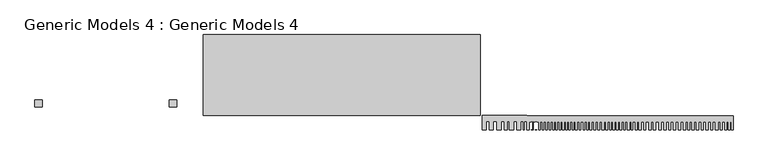
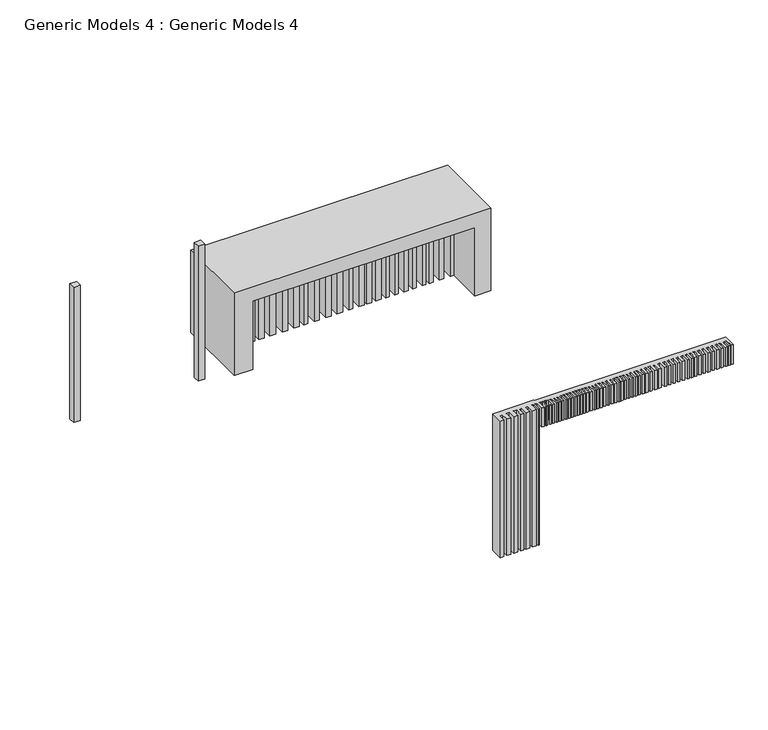
"""IFC4 building model written with IfcOpenShell, lengths in millimetres: proxy geometry, Generic Models 4 : Generic Models 4."""

from ifc_helpers import new_model, si_unit, frame, origin, place, context, project, spatial, polyline, outline, extrude, faceted_brep, source, transform, mapped, element, save


def generic_models_4_generic_models_4_29f9d9a5(model_context):
    return source(origin(), model_context, "Body", "SolidModel", [
        faceted_brep([(-8072.8951638, -14169.1466243, 3352.8), (-8072.8951638, -14169.1466243, 2880.6848502), (-8019.8245913, -14169.1466243, 2880.6848502), (-8019.8245913, -14169.1466243, 3352.8), (-3625.114323, -14169.1466243, 2880.6848502), (-3625.114323, -14169.1466243, 3352.8), (-3665.2507979, -14169.1466243, 3352.8), (-3665.2507979, -14169.1466243, 2880.6848502), (-7933.2939962, -14169.1466243, 3352.8), (-7974.3314326, -14169.1466243, 3352.8), (-7974.3314326, -14169.1466243, 2880.6848502), (-7933.2939962, -14169.1466243, 2880.6848502), (-7780.27289, -14169.1466243, 3352.8), (-7815.2998882, -14169.1466243, 3352.8), (-7815.2998882, -14169.1466243, 2880.6848502), (-7780.27289, -14169.1466243, 2880.6848502), (-7702.1357404, -14169.1466243, 3352.8), (-7737.1627385, -14169.1466243, 3352.8), (-7737.1627385, -14169.1466243, 2880.6848502), (-7702.1357404, -14169.1466243, 2880.6848502), (-7629.3873597, -14169.1466243, 3352.8), (-7664.4143578, -14169.1466243, 3352.8), (-7664.4143578, -14169.1466243, 2880.6848502), (-7629.3873597, -14169.1466243, 2880.6848502), (-7559.3333635, -14169.1466243, 3352.8), (-7591.6659771, -14169.1466243, 3352.8), (-7591.6659771, -14169.1466243, 2880.6848502), (-7559.3333635, -14169.1466243, 2880.6848502), (-7478.5018294, -14169.1466243, 3352.8), (-7516.223212, -14169.1466243, 3352.8), (-7516.223212, -14169.1466243, 2880.6848502), (-7478.5018294, -14169.1466243, 2880.6848502), (-7411.1422177, -14169.1466243, 3352.8), (-7443.4748313, -14169.1466243, 3352.8), (-7443.4748313, -14169.1466243, 2880.6848502), (-7411.1422177, -14169.1466243, 2880.6848502), (-7343.7826059, -14169.1466243, 3352.8), (-7376.1152195, -14169.1466243, 3352.8), (-7376.1152195, -14169.1466243, 2880.6848502), (-7343.7826059, -14169.1466243, 2880.6848502), (-7265.6454563, -14169.1466243, 3352.8), (-7308.7556078, -14169.1466243, 3352.8), (-7308.7556078, -14169.1466243, 2880.6848502), (-7265.6454563, -14169.1466243, 2880.6848502), (-7203.6746135, -14169.1466243, 3352.8), (-7236.0072271, -14169.1466243, 3352.8), (-7236.0072271, -14169.1466243, 2880.6848502), (-7203.6746135, -14169.1466243, 2880.6848502), (-7133.6206172, -14169.1466243, 3352.8), (-7165.9532309, -14169.1466243, 3352.8), (-7165.9532309, -14169.1466243, 2880.6848502), (-7133.6206172, -14169.1466243, 2880.6848502), (-7058.1778521, -14169.1466243, 3352.8), (-7093.2048502, -14169.1466243, 3352.8), (-7093.2048502, -14169.1466243, 2880.6848502), (-7058.1778521, -14169.1466243, 2880.6848502), (-6980.0407025, -14169.1466243, 3352.8), (-7023.150854, -14169.1466243, 3352.8), (-7023.150854, -14169.1466243, 2880.6848502), (-6980.0407025, -14169.1466243, 2880.6848502), (-6904.5979373, -14169.1466243, 3352.8), (-6942.3193199, -14169.1466243, 3352.8), (-6942.3193199, -14169.1466243, 2880.6848502), (-6904.5979373, -14169.1466243, 2880.6848502), (-6823.7664032, -14169.1466243, 3352.8), (-6858.7934013, -14169.1466243, 3352.8), (-6858.7934013, -14169.1466243, 2880.6848502), (-6823.7664032, -14169.1466243, 2880.6848502), (-6748.323638, -14169.1466243, 3352.8), (-6783.3506361, -14169.1466243, 3352.8), (-6783.3506361, -14169.1466243, 2880.6848502), (-6748.323638, -14169.1466243, 2880.6848502), (-6672.8808729, -14169.1466243, 3352.8), (-6710.6022555, -14169.1466243, 3352.8), (-6710.6022555, -14169.1466243, 2880.6848502), (-6672.8808729, -14169.1466243, 2880.6848502), (-6589.3549543, -14169.1466243, 3352.8), (-6627.0763369, -14169.1466243, 3352.8), (-6627.0763369, -14169.1466243, 2880.6848502), (-6589.3549543, -14169.1466243, 2880.6848502), (-6503.1346513, -14169.1466243, 3352.8), (-6543.5504183, -14169.1466243, 3352.8), (-6543.5504183, -14169.1466243, 2880.6848502), (-6503.1346513, -14169.1466243, 2880.6848502), (-6406.1368103, -14169.1466243, 3352.8), (-6454.6357308, -14169.1466243, 3352.8), (-6454.6357308, -14169.1466243, 2880.6848502), (-6406.1368103, -14169.1466243, 2880.6848502), (-6328.4825754, -14169.1466243, 3352.8), (-6371.1098122, -14169.1466243, 3352.8), (-6371.1098122, -14169.1466243, 2880.6848502), (-6328.4825754, -14169.1466243, 2880.6848502), (-6249.8625111, -14169.1466243, 3352.8), (-6284.8895092, -14169.1466243, 3352.8), (-6284.8895092, -14169.1466243, 2880.6848502), (-6249.8625111, -14169.1466243, 2880.6848502), (-6174.4197459, -14169.1466243, 3352.8), (-6220.2242819, -14169.1466243, 3352.8), (-6220.2242819, -14169.1466243, 2880.6848502), (-6174.4197459, -14169.1466243, 2880.6848502), (-6104.3657497, -14169.1466243, 3352.8), (-6139.3927478, -14169.1466243, 3352.8), (-6139.3927478, -14169.1466243, 2880.6848502), (-6104.3657497, -14169.1466243, 2880.6848502), (-6023.5342156, -14169.1466243, 3352.8), (-6066.6443671, -14169.1466243, 3352.8), (-6066.6443671, -14169.1466243, 2880.6848502), (-6023.5342156, -14169.1466243, 2880.6848502), (-5948.0914504, -14169.1466243, 3352.8), (-5983.1184486, -14169.1466243, 3352.8), (-5983.1184486, -14169.1466243, 2880.6848502), (-5948.0914504, -14169.1466243, 2880.6848502), (-5849.0047434, -14169.1466243, 3352.8), (-5904.9812989, -14169.1466243, 3352.8), (-5904.9812989, -14169.1466243, 2880.6848502), (-5849.0047434, -14169.1466243, 2880.6848502), (-5783.7339978, -14169.1466243, 3352.8), (-5818.7609959, -14169.1466243, 3352.8), (-5818.7609959, -14169.1466243, 2880.6848502), (-5783.7339978, -14169.1466243, 2880.6848502), (-5694.8193103, -14169.1466243, 3352.8), (-5735.2350773, -14169.1466243, 3352.8), (-5735.2350773, -14169.1466243, 2880.6848502), (-5694.8193103, -14169.1466243, 2880.6848502), (-5600.5748667, -14169.1466243, 3352.8), (-5654.4035432, -14169.1466243, 3352.8), (-5654.4035432, -14169.1466243, 2880.6848502), (-5600.5748667, -14169.1466243, 2880.6848502), (-5508.6233048, -14169.1466243, 3352.8), (-5551.3831863, -14169.1466243, 3352.8), (-5551.3831863, -14169.1466243, 2880.6848502), (-5508.6233048, -14169.1466243, 2880.6848502), (-5391.0336306, -14169.1466243, 3352.8), (-5444.4834825, -14169.1466243, 3352.8), (-5444.4834825, -14169.1466243, 2880.6848502), (-5391.0336306, -14169.1466243, 2880.6848502), (-5291.2605737, -14169.1466243, 3352.8), (-5348.273749, -14169.1466243, 3352.8), (-5348.273749, -14169.1466243, 2880.6848502), (-5291.2605737, -14169.1466243, 2880.6848502), (-5170.107576, -14169.1466243, 3352.8), (-5230.6840748, -14169.1466243, 3352.8), (-5230.6840748, -14169.1466243, 2880.6848502), (-5170.107576, -14169.1466243, 2880.6848502), (-5070.334519, -14169.1466243, 3352.8), (-5116.657724, -14169.1466243, 3352.8), (-5116.657724, -14169.1466243, 2880.6848502), (-5070.334519, -14169.1466243, 2880.6848502), (-4966.9981386, -14169.1466243, 3352.8), (-5013.3213436, -14169.1466243, 3352.8), (-5013.3213436, -14169.1466243, 2880.6848502), (-4966.9981386, -14169.1466243, 2880.6848502), (-4860.0984348, -14169.1466243, 3352.8), (-4909.9849633, -14169.1466243, 3352.8), (-4909.9849633, -14169.1466243, 2880.6848502), (-4860.0984348, -14169.1466243, 2880.6848502), (-4753.198731, -14169.1466243, 3352.8), (-4806.6485829, -14169.1466243, 3352.8), (-4806.6485829, -14169.1466243, 2880.6848502), (-4753.198731, -14169.1466243, 2880.6848502), (-4649.8623506, -14169.1466243, 3352.8), (-4696.1855556, -14169.1466243, 3352.8), (-4696.1855556, -14169.1466243, 2880.6848502), (-4649.8623506, -14169.1466243, 2880.6848502), (-4553.6526171, -14169.1466243, 3352.8), (-4603.5391456, -14169.1466243, 3352.8), (-4603.5391456, -14169.1466243, 2880.6848502), (-4553.6526171, -14169.1466243, 2880.6848502), (-4464.5695306, -14169.1466243, 3352.8), (-4510.8927356, -14169.1466243, 3352.8), (-4510.8927356, -14169.1466243, 2880.6848502), (-4464.5695306, -14169.1466243, 2880.6848502), (-4364.7964736, -14169.1466243, 3352.8), (-4418.2463256, -14169.1466243, 3352.8), (-4418.2463256, -14169.1466243, 2880.6848502), (-4364.7964736, -14169.1466243, 2880.6848502), (-4268.5867402, -14169.1466243, 3352.8), (-4314.9099452, -14169.1466243, 3352.8), (-4314.9099452, -14169.1466243, 2880.6848502), (-4268.5867402, -14169.1466243, 2880.6848502), (-4158.1237129, -14169.1466243, 3352.8), (-4218.7002117, -14169.1466243, 3352.8), (-4218.7002117, -14169.1466243, 2880.6848502), (-4158.1237129, -14169.1466243, 2880.6848502), (-4058.350656, -14169.1466243, 3352.8), (-4104.673861, -14169.1466243, 3352.8), (-4104.673861, -14169.1466243, 2880.6848502), (-4058.350656, -14169.1466243, 2880.6848502), (-3947.8876286, -14169.1466243, 3352.8), (-4004.900804, -14169.1466243, 3352.8), (-4004.900804, -14169.1466243, 2880.6848502), (-3947.8876286, -14169.1466243, 2880.6848502), (-3853.714323, -14169.1466243, 3352.8), (-3899.240517, -14169.1466243, 3352.8), (-3899.240517, -14169.1466243, 2880.6848502), (-3853.714323, -14169.1466243, 2880.6848502), (-3766.003205, -14169.1466243, 3352.8), (-3809.382795, -14169.1466243, 3352.8), (-3809.382795, -14169.1466243, 2880.6848502), (-3766.003205, -14169.1466243, 2880.6848502), (-3688.6802281, -14169.1466243, 3352.8), (-3725.7221572, -14169.1466243, 3352.8), (-3725.7221572, -14169.1466243, 2880.6848502), (-3688.6802281, -14169.1466243, 2880.6848502), (-3625.114323, -13864.3466243, 3352.8), (-3625.114323, -13864.3466243, 2880.6848502), (-8072.8951638, -13864.3466243, 2880.6848502), (-8072.8951638, -13864.3466243, 3352.8), (-8072.8951638, -13854.1538163, 3352.8), (-9031.8508279, -13854.1538163, 3352.8), (-9031.8508279, -14158.9538163, 3352.8), (-8947.3984101, -14158.9538163, 3352.8), (-8947.3984101, -13981.1538163, 3352.8), (-8878.843385, -13981.1538163, 3352.8), (-8878.843385, -14158.9538163, 3352.8), (-8791.591535, -14158.9538163, 3352.8), (-8791.591535, -13981.1538163, 3352.8), (-8723.0365099, -13981.1538163, 3352.8), (-8723.0365099, -14158.9538163, 3352.8), (-8623.3201098, -14158.9538163, 3352.8), (-8623.3201098, -13981.1538163, 3352.8), (-8552.3729958, -13981.1538163, 3352.8), (-8552.3729958, -14158.9538163, 3352.8), (-8491.4762732, -14158.9538163, 3352.8), (-8491.4762732, -13981.1538163, 3352.8), (-8443.291009, -13981.1538163, 3352.8), (-8443.291009, -14158.9538163, 3352.8), (-8349.8068839, -14158.9538163, 3352.8), (-8349.8068839, -13981.1538163, 3352.8), (-8287.4841338, -13981.1538163, 3352.8), (-8287.4841338, -14158.9538163, 3352.8), (-8200.8633881, -14158.9538163, 3352.8), (-8200.8633881, -13981.1538163, 3352.8), (-8151.7037606, -13981.1538163, 3352.8), (-8151.7037606, -14158.9538163, 3352.8), (-8123.0396657, -14158.9538163, 3352.8), (-8123.0396657, -13981.1538163, 3352.8), (-8072.8951638, -13981.1538163, 3352.8), (-8019.8245913, -13981.1538163, 3352.8), (-8009.5759038, -13981.1538163, 3352.8), (-8009.5759038, -13991.3466243, 3352.8), (-8001.1139413, -13991.3466243, 3352.8), (-8001.1139413, -13981.1538163, 3352.8), (-7990.6394273, -13981.1538163, 3352.8), (-7990.6394273, -13991.3466243, 3352.8), (-7974.3314326, -13991.3466243, 3352.8), (-7974.3314326, -13981.1538163, 3352.8), (-7946.1776726, -13981.1538163, 3352.8), (-7946.1776726, -14158.9538163, 3352.8), (-7974.3314326, -14158.9538163, 3352.8), (-7933.2939962, -13981.1538163, 3352.8), (-7908.7622496, -13981.1538163, 3352.8), (-7908.7622496, -13991.3466243, 3352.8), (-7885.3328194, -13991.3466243, 3352.8), (-7885.3328194, -13981.1538163, 3352.8), (-7854.214323, -13981.1538163, 3352.8), (-7854.214323, -13991.3466243, 3352.8), (-7815.2998882, -13991.3466243, 3352.8), (-7780.27289, -13991.3466243, 3352.8), (-7737.1627385, -13991.3466243, 3352.8), (-7702.1357404, -13991.3466243, 3352.8), (-7664.4143578, -13991.3466243, 3352.8), (-7629.3873597, -13991.3466243, 3352.8), (-7591.6659771, -13991.3466243, 3352.8), (-7559.3333635, -13991.3466243, 3352.8), (-7516.223212, -13991.3466243, 3352.8), (-7478.5018294, -13991.3466243, 3352.8), (-7443.4748313, -13991.3466243, 3352.8), (-7411.1422177, -13991.3466243, 3352.8), (-7376.1152195, -13991.3466243, 3352.8), (-7343.7826059, -13991.3466243, 3352.8), (-7308.7556078, -13991.3466243, 3352.8), (-7265.6454563, -13991.3466243, 3352.8), (-7236.0072271, -13991.3466243, 3352.8), (-7203.6746135, -13991.3466243, 3352.8), (-7165.9532309, -13991.3466243, 3352.8), (-7133.6206172, -13991.3466243, 3352.8), (-7093.2048502, -13991.3466243, 3352.8), (-7058.1778521, -13991.3466243, 3352.8), (-7023.150854, -13991.3466243, 3352.8), (-6980.0407025, -13991.3466243, 3352.8), (-6942.3193199, -13991.3466243, 3352.8), (-6904.5979373, -13991.3466243, 3352.8), (-6858.7934013, -13991.3466243, 3352.8), (-6823.7664032, -13991.3466243, 3352.8), (-6783.3506361, -13991.3466243, 3352.8), (-6748.323638, -13991.3466243, 3352.8), (-6710.6022555, -13991.3466243, 3352.8), (-6672.8808729, -13991.3466243, 3352.8), (-6627.0763369, -13991.3466243, 3352.8), (-6589.3549543, -13991.3466243, 3352.8), (-6543.5504183, -13991.3466243, 3352.8), (-6503.1346513, -13991.3466243, 3352.8), (-6454.6357308, -13991.3466243, 3352.8), (-6406.1368103, -13991.3466243, 3352.8), (-6371.1098122, -13991.3466243, 3352.8), (-6328.4825754, -13991.3466243, 3352.8), (-6284.8895092, -13991.3466243, 3352.8), (-6249.8625111, -13991.3466243, 3352.8), (-6220.2242819, -13991.3466243, 3352.8), (-6174.4197459, -13991.3466243, 3352.8), (-6139.3927478, -13991.3466243, 3352.8), (-6104.3657497, -13991.3466243, 3352.8), (-6066.6443671, -13991.3466243, 3352.8), (-6023.5342156, -13991.3466243, 3352.8), (-5983.1184486, -13991.3466243, 3352.8), (-5948.0914504, -13991.3466243, 3352.8), (-5904.9812989, -13991.3466243, 3352.8), (-5849.0047434, -13991.3466243, 3352.8), (-5818.7609959, -13991.3466243, 3352.8), (-5783.7339978, -13991.3466243, 3352.8), (-5735.2350773, -13991.3466243, 3352.8), (-5694.8193103, -13991.3466243, 3352.8), (-5654.4035432, -13991.3466243, 3352.8), (-5600.5748667, -13991.3466243, 3352.8), (-5551.3831863, -13991.3466243, 3352.8), (-5508.6233048, -13991.3466243, 3352.8), (-5444.4834825, -13991.3466243, 3352.8), (-5391.0336306, -13991.3466243, 3352.8), (-5348.273749, -13991.3466243, 3352.8), (-5291.2605737, -13991.3466243, 3352.8), (-5230.6840748, -13991.3466243, 3352.8), (-5170.107576, -13991.3466243, 3352.8), (-5116.657724, -13991.3466243, 3352.8), (-5070.334519, -13991.3466243, 3352.8), (-5013.3213436, -13991.3466243, 3352.8), (-4966.9981386, -13991.3466243, 3352.8), (-4909.9849633, -13991.3466243, 3352.8), (-4860.0984348, -13991.3466243, 3352.8), (-4806.6485829, -13991.3466243, 3352.8), (-4753.198731, -13991.3466243, 3352.8), (-4696.1855556, -13991.3466243, 3352.8), (-4649.8623506, -13991.3466243, 3352.8), (-4603.5391456, -13991.3466243, 3352.8), (-4553.6526171, -13991.3466243, 3352.8), (-4510.8927356, -13991.3466243, 3352.8), (-4464.5695306, -13991.3466243, 3352.8), (-4418.2463256, -13991.3466243, 3352.8), (-4364.7964736, -13991.3466243, 3352.8), (-4314.9099452, -13991.3466243, 3352.8), (-4268.5867402, -13991.3466243, 3352.8), (-4218.7002117, -13991.3466243, 3352.8), (-4158.1237129, -13991.3466243, 3352.8), (-4104.673861, -13991.3466243, 3352.8), (-4058.350656, -13991.3466243, 3352.8), (-4004.900804, -13991.3466243, 3352.8), (-3947.8876286, -13991.3466243, 3352.8), (-3899.240517, -13991.3466243, 3352.8), (-3853.714323, -13991.3466243, 3352.8), (-3809.382795, -13991.3466243, 3352.8), (-3766.003205, -13991.3466243, 3352.8), (-3725.7221572, -13991.3466243, 3352.8), (-3688.6802281, -13991.3466243, 3352.8), (-3665.2507979, -13991.3466243, 3352.8), (-8072.8951638, -13981.1538163, 2880.6848502), (-3665.2507979, -13991.3466243, 2880.6848502), (-3688.6802281, -13991.3466243, 2880.6848502), (-3725.7221572, -13991.3466243, 2880.6848502), (-3766.003205, -13991.3466243, 2880.6848502), (-3809.382795, -13991.3466243, 2880.6848502), (-3853.714323, -13991.3466243, 2880.6848502), (-3899.240517, -13991.3466243, 2880.6848502), (-3947.8876286, -13991.3466243, 2880.6848502), (-4004.900804, -13991.3466243, 2880.6848502), (-4058.350656, -13991.3466243, 2880.6848502), (-4104.673861, -13991.3466243, 2880.6848502), (-4158.1237129, -13991.3466243, 2880.6848502), (-4218.7002117, -13991.3466243, 2880.6848502), (-4268.5867402, -13991.3466243, 2880.6848502), (-4314.9099452, -13991.3466243, 2880.6848502), (-4364.7964736, -13991.3466243, 2880.6848502), (-4418.2463256, -13991.3466243, 2880.6848502), (-4464.5695306, -13991.3466243, 2880.6848502), (-4510.8927356, -13991.3466243, 2880.6848502), (-4553.6526171, -13991.3466243, 2880.6848502), (-4603.5391456, -13991.3466243, 2880.6848502), (-4649.8623506, -13991.3466243, 2880.6848502), (-4696.1855556, -13991.3466243, 2880.6848502), (-4753.198731, -13991.3466243, 2880.6848502), (-4806.6485829, -13991.3466243, 2880.6848502), (-4860.0984348, -13991.3466243, 2880.6848502), (-4909.9849633, -13991.3466243, 2880.6848502), (-4966.9981386, -13991.3466243, 2880.6848502), (-5013.3213436, -13991.3466243, 2880.6848502), (-5070.334519, -13991.3466243, 2880.6848502), (-5116.657724, -13991.3466243, 2880.6848502), (-5170.107576, -13991.3466243, 2880.6848502), (-5230.6840748, -13991.3466243, 2880.6848502), (-5291.2605737, -13991.3466243, 2880.6848502), (-5348.273749, -13991.3466243, 2880.6848502), (-5391.0336306, -13991.3466243, 2880.6848502), (-5444.4834825, -13991.3466243, 2880.6848502), (-5508.6233048, -13991.3466243, 2880.6848502), (-5551.3831863, -13991.3466243, 2880.6848502), (-5600.5748667, -13991.3466243, 2880.6848502), (-5654.4035432, -13991.3466243, 2880.6848502), (-5694.8193103, -13991.3466243, 2880.6848502), (-5735.2350773, -13991.3466243, 2880.6848502), (-5783.7339978, -13991.3466243, 2880.6848502), (-5818.7609959, -13991.3466243, 2880.6848502), (-5849.0047434, -13991.3466243, 2880.6848502), (-5904.9812989, -13991.3466243, 2880.6848502), (-5948.0914504, -13991.3466243, 2880.6848502), (-5983.1184486, -13991.3466243, 2880.6848502), (-6023.5342156, -13991.3466243, 2880.6848502), (-6066.6443671, -13991.3466243, 2880.6848502), (-6104.3657497, -13991.3466243, 2880.6848502), (-6139.3927478, -13991.3466243, 2880.6848502), (-6174.4197459, -13991.3466243, 2880.6848502), (-6220.2242819, -13991.3466243, 2880.6848502), (-6249.8625111, -13991.3466243, 2880.6848502), (-6284.8895092, -13991.3466243, 2880.6848502), (-6328.4825754, -13991.3466243, 2880.6848502), (-6371.1098122, -13991.3466243, 2880.6848502), (-6406.1368103, -13991.3466243, 2880.6848502), (-6454.6357308, -13991.3466243, 2880.6848502), (-6503.1346513, -13991.3466243, 2880.6848502), (-6543.5504183, -13991.3466243, 2880.6848502), (-6589.3549543, -13991.3466243, 2880.6848502), (-6627.0763369, -13991.3466243, 2880.6848502), (-6672.8808729, -13991.3466243, 2880.6848502), (-6710.6022555, -13991.3466243, 2880.6848502), (-6748.323638, -13991.3466243, 2880.6848502), (-6783.3506361, -13991.3466243, 2880.6848502), (-6823.7664032, -13991.3466243, 2880.6848502), (-6858.7934013, -13991.3466243, 2880.6848502), (-6904.5979373, -13991.3466243, 2880.6848502), (-6942.3193199, -13991.3466243, 2880.6848502), (-6980.0407025, -13991.3466243, 2880.6848502), (-7023.150854, -13991.3466243, 2880.6848502), (-7058.1778521, -13991.3466243, 2880.6848502), (-7093.2048502, -13991.3466243, 2880.6848502), (-7133.6206172, -13991.3466243, 2880.6848502), (-7165.9532309, -13991.3466243, 2880.6848502), (-7203.6746135, -13991.3466243, 2880.6848502), (-7236.0072271, -13991.3466243, 2880.6848502), (-7265.6454563, -13991.3466243, 2880.6848502), (-7308.7556078, -13991.3466243, 2880.6848502), (-7343.7826059, -13991.3466243, 2880.6848502), (-7376.1152195, -13991.3466243, 2880.6848502), (-7411.1422177, -13991.3466243, 2880.6848502), (-7443.4748313, -13991.3466243, 2880.6848502), (-7478.5018294, -13991.3466243, 2880.6848502), (-7516.223212, -13991.3466243, 2880.6848502), (-7559.3333635, -13991.3466243, 2880.6848502), (-7591.6659771, -13991.3466243, 2880.6848502), (-7629.3873597, -13991.3466243, 2880.6848502), (-7664.4143578, -13991.3466243, 2880.6848502), (-7702.1357404, -13991.3466243, 2880.6848502), (-7737.1627385, -13991.3466243, 2880.6848502), (-7780.27289, -13991.3466243, 2880.6848502), (-7815.2998882, -13991.3466243, 2880.6848502), (-7854.214323, -13991.3466243, 2880.6848502), (-7854.214323, -13981.1538163, 2880.6848502), (-7885.3328194, -13981.1538163, 2880.6848502), (-7885.3328194, -13991.3466243, 2880.6848502), (-7908.7622496, -13991.3466243, 2880.6848502), (-7908.7622496, -13981.1538163, 2880.6848502), (-7933.2939962, -13981.1538163, 2880.6848502), (-7974.3314326, -14158.9538163, 2880.6848502), (-7946.1776726, -14158.9538163, 2880.6848502), (-7946.1776726, -13981.1538163, 2880.6848502), (-7974.3314326, -13981.1538163, 2880.6848502), (-7974.3314326, -13991.3466243, 2880.6848502), (-7990.6394273, -13991.3466243, 2880.6848502), (-7990.6394273, -13981.1538163, 2880.6848502), (-8001.1139413, -13981.1538163, 2880.6848502), (-8001.1139413, -13991.3466243, 2880.6848502), (-8009.5759038, -13991.3466243, 2880.6848502), (-8009.5759038, -13981.1538163, 2880.6848502), (-8019.8245913, -13981.1538163, 2880.6848502), (-9031.8508279, -14158.9538163, 0.0), (-8947.3984101, -14158.9538163, 0.0), (-8151.7037606, -14158.9538163, 0.0), (-8123.0396657, -14158.9538163, 0.0), (-8287.4841338, -14158.9538163, 0.0), (-8200.8633881, -14158.9538163, 0.0), (-8443.291009, -14158.9538163, 0.0), (-8349.8068839, -14158.9538163, 0.0), (-8552.3729958, -14158.9538163, 0.0), (-8491.4762732, -14158.9538163, 0.0), (-8723.0365099, -14158.9538163, 0.0), (-8623.3201098, -14158.9538163, 0.0), (-8878.843385, -14158.9538163, 0.0), (-8791.591535, -14158.9538163, 0.0), (-9031.8508279, -13854.1538163, 0.0), (-8072.8951638, -13854.1538163, 0.0), (-8072.8951638, -13981.1538163, 0.0), (-8123.0396657, -13981.1538163, 0.0), (-8151.7037606, -13981.1538163, 0.0), (-8200.8633881, -13981.1538163, 0.0), (-8287.4841338, -13981.1538163, 0.0), (-8349.8068839, -13981.1538163, 0.0), (-8443.291009, -13981.1538163, 0.0), (-8491.4762732, -13981.1538163, 0.0), (-8552.3729958, -13981.1538163, 0.0), (-8623.3201098, -13981.1538163, 0.0), (-8723.0365099, -13981.1538163, 0.0), (-8791.591535, -13981.1538163, 0.0), (-8878.843385, -13981.1538163, 0.0), (-8947.3984101, -13981.1538163, 0.0)], [[[0, 1, 2, 3]], [[4, 5, 6, 7]], [[8, 9, 10, 11]], [[12, 13, 14, 15]], [[16, 17, 18, 19]], [[20, 21, 22, 23]], [[24, 25, 26, 27]], [[28, 29, 30, 31]], [[32, 33, 34, 35]], [[36, 37, 38, 39]], [[40, 41, 42, 43]], [[44, 45, 46, 47]], [[48, 49, 50, 51]], [[52, 53, 54, 55]], [[56, 57, 58, 59]], [[60, 61, 62, 63]], [[64, 65, 66, 67]], [[68, 69, 70, 71]], [[72, 73, 74, 75]], [[76, 77, 78, 79]], [[80, 81, 82, 83]], [[84, 85, 86, 87]], [[88, 89, 90, 91]], [[92, 93, 94, 95]], [[96, 97, 98, 99]], [[100, 101, 102, 103]], [[104, 105, 106, 107]], [[108, 109, 110, 111]], [[112, 113, 114, 115]], [[116, 117, 118, 119]], [[120, 121, 122, 123]], [[124, 125, 126, 127]], [[128, 129, 130, 131]], [[132, 133, 134, 135]], [[136, 137, 138, 139]], [[140, 141, 142, 143]], [[144, 145, 146, 147]], [[148, 149, 150, 151]], [[152, 153, 154, 155]], [[156, 157, 158, 159]], [[160, 161, 162, 163]], [[164, 165, 166, 167]], [[168, 169, 170, 171]], [[172, 173, 174, 175]], [[176, 177, 178, 179]], [[180, 181, 182, 183]], [[184, 185, 186, 187]], [[188, 189, 190, 191]], [[192, 193, 194, 195]], [[196, 197, 198, 199]], [[200, 201, 202, 203]], [[204, 205, 206, 207]], [[204, 207, 208, 209, 210, 211, 212, 213, 214, 215, 216, 217, 218, 219, 220, 221, 222, 223, 224, 225, 226, 227, 228, 229, 230, 231, 232, 233, 234, 235, 236, 237, 0, 3, 238, 239, 240, 241, 242, 243, 244, 245, 246, 247, 248, 249, 9, 8, 250, 251, 252, 253, 254, 255, 256, 257, 13, 12, 258, 259, 17, 16, 260, 261, 21, 20, 262, 263, 25, 24, 264, 265, 29, 28, 266, 267, 33, 32, 268, 269, 37, 36, 270, 271, 41, 40, 272, 273, 45, 44, 274, 275, 49, 48, 276, 277, 53, 52, 278, 279, 57, 56, 280, 281, 61, 60, 282, 283, 65, 64, 284, 285, 69, 68, 286, 287, 73, 72, 288, 289, 77, 76, 290, 291, 81, 80, 292, 293, 85, 84, 294, 295, 89, 88, 296, 297, 93, 92, 298, 299, 97, 96, 300, 301, 101, 100, 302, 303, 105, 104, 304, 305, 109, 108, 306, 307, 113, 112, 308, 309, 117, 116, 310, 311, 121, 120, 312, 313, 125, 124, 314, 315, 129, 128, 316, 317, 133, 132, 318, 319, 137, 136, 320, 321, 141, 140, 322, 323, 145, 144, 324, 325, 149, 148, 326, 327, 153, 152, 328, 329, 157, 156, 330, 331, 161, 160, 332, 333, 165, 164, 334, 335, 169, 168, 336, 337, 173, 172, 338, 339, 177, 176, 340, 341, 181, 180, 342, 343, 185, 184, 344, 345, 189, 188, 346, 347, 193, 192, 348, 349, 197, 196, 350, 351, 201, 200, 352, 353, 6, 5]], [[1, 0, 237, 354]], [[206, 205, 4, 7, 355, 356, 203, 202, 357, 358, 199, 198, 359, 360, 195, 194, 361, 362, 191, 190, 363, 364, 187, 186, 365, 366, 183, 182, 367, 368, 179, 178, 369, 370, 175, 174, 371, 372, 171, 170, 373, 374, 167, 166, 375, 376, 163, 162, 377, 378, 159, 158, 379, 380, 155, 154, 381, 382, 151, 150, 383, 384, 147, 146, 385, 386, 143, 142, 387, 388, 139, 138, 389, 390, 135, 134, 391, 392, 131, 130, 393, 394, 127, 126, 395, 396, 123, 122, 397, 398, 119, 118, 399, 400, 115, 114, 401, 402, 111, 110, 403, 404, 107, 106, 405, 406, 103, 102, 407, 408, 99, 98, 409, 410, 95, 94, 411, 412, 91, 90, 413, 414, 87, 86, 415, 416, 83, 82, 417, 418, 79, 78, 419, 420, 75, 74, 421, 422, 71, 70, 423, 424, 67, 66, 425, 426, 63, 62, 427, 428, 59, 58, 429, 430, 55, 54, 431, 432, 51, 50, 433, 434, 47, 46, 435, 436, 43, 42, 437, 438, 39, 38, 439, 440, 35, 34, 441, 442, 31, 30, 443, 444, 27, 26, 445, 446, 23, 22, 447, 448, 19, 18, 449, 450, 15, 14, 451, 452, 453, 454, 455, 456, 457, 458, 11, 10, 459, 460, 461, 462, 463, 464, 465, 466, 467, 468, 469, 470, 2, 1, 354]], [[5, 4, 205, 204]], [[210, 471, 472, 211]], [[473, 474, 235, 234]], [[475, 476, 231, 230]], [[477, 478, 227, 226]], [[479, 480, 223, 222]], [[481, 482, 219, 218]], [[483, 484, 215, 214]], [[485, 209, 208, 486]], [[485, 486, 487, 488, 474, 473, 489, 490, 476, 475, 491, 492, 478, 477, 493, 494, 480, 479, 495, 496, 482, 481, 497, 498, 484, 483, 499, 500, 472, 471]], [[486, 208, 207, 206, 354, 487]], [[471, 210, 209, 485]], [[236, 488, 487, 354, 237]], [[489, 233, 232, 490]], [[228, 492, 491, 229]], [[224, 494, 493, 225]], [[220, 496, 495, 221]], [[216, 498, 497, 217]], [[212, 500, 499, 213]], [[254, 454, 453, 255]], [[457, 251, 250, 458]], [[461, 247, 246, 462]], [[242, 466, 465, 243]], [[469, 239, 238, 470]], [[248, 460, 459, 249]], [[488, 236, 235, 474]], [[490, 232, 231, 476]], [[233, 489, 473, 234]], [[255, 453, 452, 256]], [[454, 254, 253, 455]], [[458, 250, 8, 11]], [[251, 457, 456, 252]], [[462, 246, 245, 463]], [[247, 461, 460, 248]], [[243, 465, 464, 244]], [[466, 242, 241, 467]], [[470, 238, 3, 2]], [[239, 469, 468, 240]], [[229, 491, 475, 230]], [[492, 228, 227, 478]], [[225, 493, 477, 226]], [[494, 224, 223, 480]], [[221, 495, 479, 222]], [[496, 220, 219, 482]], [[217, 497, 481, 218]], [[498, 216, 215, 484]], [[213, 499, 483, 214]], [[500, 212, 211, 472]], [[241, 240, 468, 467]], [[245, 244, 464, 463]], [[253, 252, 456, 455]], [[451, 257, 256, 452]], [[258, 450, 449, 259]], [[260, 448, 447, 261]], [[262, 446, 445, 263]], [[264, 444, 443, 265]], [[266, 442, 441, 267]], [[268, 440, 439, 269]], [[270, 438, 437, 271]], [[272, 436, 435, 273]], [[274, 434, 433, 275]], [[276, 432, 431, 277]], [[278, 430, 429, 279]], [[280, 428, 427, 281]], [[282, 426, 425, 283]], [[284, 424, 423, 285]], [[286, 422, 421, 287]], [[288, 420, 419, 289]], [[290, 418, 417, 291]], [[292, 416, 415, 293]], [[294, 414, 413, 295]], [[296, 412, 411, 297]], [[298, 410, 409, 299]], [[300, 408, 407, 301]], [[302, 406, 405, 303]], [[304, 404, 403, 305]], [[306, 402, 401, 307]], [[308, 400, 399, 309]], [[310, 398, 397, 311]], [[312, 396, 395, 313]], [[314, 394, 393, 315]], [[316, 392, 391, 317]], [[318, 390, 389, 319]], [[320, 388, 387, 321]], [[322, 386, 385, 323]], [[324, 384, 383, 325]], [[326, 382, 381, 327]], [[328, 380, 379, 329]], [[330, 378, 377, 331]], [[332, 376, 375, 333]], [[334, 374, 373, 335]], [[336, 372, 371, 337]], [[338, 370, 369, 339]], [[340, 368, 367, 341]], [[342, 366, 365, 343]], [[344, 364, 363, 345]], [[346, 362, 361, 347]], [[348, 360, 359, 349]], [[350, 358, 357, 351]], [[352, 356, 355, 353]], [[10, 9, 249, 459]], [[257, 451, 14, 13]], [[259, 449, 18, 17]], [[450, 258, 12, 15]], [[261, 447, 22, 21]], [[448, 260, 16, 19]], [[263, 445, 26, 25]], [[446, 262, 20, 23]], [[265, 443, 30, 29]], [[444, 264, 24, 27]], [[267, 441, 34, 33]], [[442, 266, 28, 31]], [[269, 439, 38, 37]], [[440, 268, 32, 35]], [[271, 437, 42, 41]], [[438, 270, 36, 39]], [[273, 435, 46, 45]], [[436, 272, 40, 43]], [[275, 433, 50, 49]], [[434, 274, 44, 47]], [[277, 431, 54, 53]], [[432, 276, 48, 51]], [[279, 429, 58, 57]], [[430, 278, 52, 55]], [[281, 427, 62, 61]], [[428, 280, 56, 59]], [[283, 425, 66, 65]], [[426, 282, 60, 63]], [[285, 423, 70, 69]], [[424, 284, 64, 67]], [[287, 421, 74, 73]], [[422, 286, 68, 71]], [[289, 419, 78, 77]], [[420, 288, 72, 75]], [[291, 417, 82, 81]], [[418, 290, 76, 79]], [[293, 415, 86, 85]], [[416, 292, 80, 83]], [[295, 413, 90, 89]], [[414, 294, 84, 87]], [[297, 411, 94, 93]], [[412, 296, 88, 91]], [[299, 409, 98, 97]], [[410, 298, 92, 95]], [[301, 407, 102, 101]], [[408, 300, 96, 99]], [[303, 405, 106, 105]], [[406, 302, 100, 103]], [[305, 403, 110, 109]], [[404, 304, 104, 107]], [[307, 401, 114, 113]], [[402, 306, 108, 111]], [[309, 399, 118, 117]], [[400, 308, 112, 115]], [[311, 397, 122, 121]], [[398, 310, 116, 119]], [[313, 395, 126, 125]], [[396, 312, 120, 123]], [[315, 393, 130, 129]], [[394, 314, 124, 127]], [[317, 391, 134, 133]], [[392, 316, 128, 131]], [[319, 389, 138, 137]], [[390, 318, 132, 135]], [[321, 387, 142, 141]], [[388, 320, 136, 139]], [[323, 385, 146, 145]], [[386, 322, 140, 143]], [[325, 383, 150, 149]], [[384, 324, 144, 147]], [[327, 381, 154, 153]], [[382, 326, 148, 151]], [[329, 379, 158, 157]], [[380, 328, 152, 155]], [[331, 377, 162, 161]], [[378, 330, 156, 159]], [[333, 375, 166, 165]], [[376, 332, 160, 163]], [[335, 373, 170, 169]], [[374, 334, 164, 167]], [[337, 371, 174, 173]], [[372, 336, 168, 171]], [[339, 369, 178, 177]], [[370, 338, 172, 175]], [[341, 367, 182, 181]], [[368, 340, 176, 179]], [[343, 365, 186, 185]], [[366, 342, 180, 183]], [[345, 363, 190, 189]], [[364, 344, 184, 187]], [[347, 361, 194, 193]], [[362, 346, 188, 191]], [[349, 359, 198, 197]], [[360, 348, 192, 195]], [[351, 357, 202, 201]], [[358, 350, 196, 199]], [[353, 355, 7, 6]], [[356, 352, 200, 203]]]),
        faceted_brep([(-7854.214323, -14169.1466243, 3352.8), (-7885.3328194, -14169.1466243, 3352.8), (-7885.3328194, -14169.1466243, 2880.6848502), (-7854.214323, -14169.1466243, 2880.6848502), (-7854.214323, -14158.9538163, 3352.8), (-7885.3328194, -14158.9538163, 3352.8), (-7885.3328194, -14158.9538163, 2880.6848502), (-7854.214323, -14158.9538163, 2880.6848502)], [[[0, 1, 2, 3]], [[4, 5, 1, 0]], [[6, 7, 3, 2]], [[5, 4, 7, 6]], [[2, 1, 5, 6]], [[0, 3, 7, 4]]]),
        extrude(outline(polyline([(-15770.4931546, -13513.5648332), (-15618.0931546, -13513.5648332), (-15618.0931546, -13665.9648332), (-15770.4931546, -13665.9648332), (-15770.4931546, -13513.5648332)])), frame((0.0, 0.0, 6400.8), z_axis=(0.0, 0.0, 1.0), x_axis=(1.0, 0.0, 0.0)), (0.0, 0.0, 1.0), 3323.8345251),
        extrude(outline(polyline([(-18510.2549486, -13665.9648332), (-18669.7002465, -13665.9648332), (-18669.7002465, -13513.5648332), (-18510.2549486, -13513.5648332), (-18510.2549486, -13665.9648332)])), frame((0.0, 0.0, 6400.8), z_axis=(0.0, 0.0, 1.0), x_axis=(1.0, 0.0, 0.0)), (0.0, 0.0, 1.0), 3323.8345251),
        faceted_brep([(-15045.589323, -13854.1538163, 8426.7048313), (-9073.414323, -13854.1538163, 8426.7048313), (-9073.414323, -12110.5517145, 8426.7048313), (-15045.589323, -12110.5517145, 8426.7048313), (-15045.589323, -13854.1538163, 6400.8), (-15045.589323, -12110.5517145, 6400.8), (-9073.414323, -12110.5517145, 6400.8), (-9073.414323, -13854.1538163, 6400.8), (-9448.3676558, -13854.1538163, 6400.8), (-9448.3676558, -13015.9538163, 6400.8), (-9539.2812482, -13015.9538163, 6400.8), (-9539.2812482, -12406.3538163, 6400.8), (-9690.3788117, -12406.3538163, 6400.8), (-9690.3788117, -13015.9538163, 6400.8), (-9786.5318067, -13015.9538163, 6400.8), (-9786.5318067, -12406.3538163, 6400.8), (-9930.7612992, -12406.3538163, 6400.8), (-9930.7612992, -13015.9538163, 6400.8), (-10020.0462232, -13015.9538163, 6400.8), (-10020.0462232, -12406.3538163, 6400.8), (-10109.3311471, -12406.3538163, 6400.8), (-10109.3311471, -13015.9538163, 6400.8), (-10191.7479999, -13015.9538163, 6400.8), (-10191.7479999, -12406.3538163, 6400.8), (-10322.2413503, -12406.3538163, 6400.8), (-10322.2413503, -13015.9538163, 6400.8), (-10406.914323, -13015.9538163, 6400.8), (-10406.914323, -12406.3538163, 6400.8), (-10514.5473403, -12406.3538163, 6400.8), (-10514.5473403, -13015.9538163, 6400.8), (-10617.5684064, -13015.9538163, 6400.8), (-10617.5684064, -12406.3538163, 6400.8), (-10741.1936856, -12406.3538163, 6400.8), (-10741.1936856, -13015.9538163, 6400.8), (-10830.4786096, -13015.9538163, 6400.8), (-10830.4786096, -12406.3538163, 6400.8), (-10954.1038889, -12406.3538163, 6400.8), (-10954.1038889, -13015.9538163, 6400.8), (-11036.5207417, -13015.9538163, 6400.8), (-11036.5207417, -12406.3538163, 6400.8), (-11139.5418078, -12406.3538163, 6400.8), (-11139.5418078, -13015.9538163, 6400.8), (-11263.1670871, -13015.9538163, 6400.8), (-11263.1670871, -12406.3538163, 6400.8), (-11366.1881531, -12406.3538163, 6400.8), (-11366.1881531, -13015.9538163, 6400.8), (-11473.714323, -13015.9538163, 6400.8), (-11473.714323, -12406.3538163, 6400.8), (-11537.5509858, -12406.3538163, 6400.8), (-11537.5509858, -13015.9538163, 6400.8), (-11663.9234935, -13015.9538163, 6400.8), (-11663.9234935, -12406.3538163, 6400.8), (-11806.0925647, -12406.3538163, 6400.8), (-11806.0925647, -13015.9538163, 6400.8), (-11900.8719455, -13015.9538163, 6400.8), (-11900.8719455, -12406.3538163, 6400.8), (-12029.4909894, -12406.3538163, 6400.8), (-12029.4909894, -13015.9538163, 6400.8), (-12177.3118061, -13015.9538163, 6400.8), (-12177.3118061, -12406.3538163, 6400.8), (-12303.6843138, -12406.3538163, 6400.8), (-12303.6843138, -13015.9538163, 6400.8), (-12430.0568215, -13015.9538163, 6400.8), (-12430.0568215, -12406.3538163, 6400.8), (-12580.1241744, -12406.3538163, 6400.8), (-12580.1241744, -13015.9538163, 6400.8), (-12698.5984004, -13015.9538163, 6400.8), (-12698.5984004, -12406.3538163, 6400.8), (-12845.314323, -12406.3538163, 6400.8), (-12845.314323, -13015.9538163, 6400.8), (-12943.4451341, -13015.9538163, 6400.8), (-12943.4451341, -12406.3538163, 6400.8), (-13046.9126248, -12406.3538163, 6400.8), (-13046.9126248, -13015.9538163, 6400.8), (-13174.0749606, -13015.9538163, 6400.8), (-13174.0749606, -12406.3538163, 6400.8), (-13319.4033445, -12406.3538163, 6400.8), (-13319.4033445, -13015.9538163, 6400.8), (-13446.5656804, -13015.9538163, 6400.8), (-13446.5656804, -12406.3538163, 6400.8), (-13591.8940643, -12406.3538163, 6400.8), (-13591.8940643, -13015.9538163, 6400.8), (-13728.1394241, -13015.9538163, 6400.8), (-13728.1394241, -12406.3538163, 6400.8), (-13855.30176, -12406.3538163, 6400.8), (-13855.30176, -13015.9538163, 6400.8), (-13982.4640959, -13015.9538163, 6400.8), (-13982.4640959, -12406.3538163, 6400.8), (-14082.3773598, -12406.3538163, 6400.8), (-14082.3773598, -13015.9538163, 6400.8), (-14236.7887677, -13015.9538163, 6400.8), (-14236.7887677, -12406.3538163, 6400.8), (-14354.8680796, -12406.3538163, 6400.8), (-14354.8680796, -13015.9538163, 6400.8), (-14496.314323, -13015.9538163, 6400.8), (-14496.314323, -12406.3538163, 6400.8), (-14610.614323, -12406.3538163, 6400.8), (-14610.614323, -13854.1538163, 6400.8), (-14610.614323, -13854.1538163, 8076.8019897), (-9448.3676558, -13854.1538163, 8076.8019897), (-9690.3788117, -13015.9538163, 8076.8019897), (-9786.5318067, -13015.9538163, 8076.8019897), (-9930.7612992, -13015.9538163, 8076.8019897), (-10020.0462232, -13015.9538163, 8076.8019897), (-10109.3311471, -13015.9538163, 8076.8019897), (-10191.7479999, -13015.9538163, 8076.8019897), (-10322.2413503, -13015.9538163, 8076.8019897), (-10406.914323, -13015.9538163, 8076.8019897), (-10514.5473403, -13015.9538163, 8076.8019897), (-10617.5684064, -13015.9538163, 8076.8019897), (-10741.1936856, -13015.9538163, 8076.8019897), (-10830.4786096, -13015.9538163, 8076.8019897), (-10954.1038889, -13015.9538163, 8076.8019897), (-11036.5207417, -13015.9538163, 8076.8019897), (-11139.5418078, -13015.9538163, 8076.8019897), (-11263.1670871, -13015.9538163, 8076.8019897), (-11366.1881531, -13015.9538163, 8076.8019897), (-11473.714323, -13015.9538163, 8076.8019897), (-11537.5509858, -13015.9538163, 8076.8019897), (-11663.9234935, -13015.9538163, 8076.8019897), (-11806.0925647, -13015.9538163, 8076.8019897), (-11900.8719455, -13015.9538163, 8076.8019897), (-12029.4909894, -13015.9538163, 8076.8019897), (-12177.3118061, -13015.9538163, 8076.8019897), (-12303.6843138, -13015.9538163, 8076.8019897), (-12430.0568215, -13015.9538163, 8076.8019897), (-12580.1241744, -13015.9538163, 8076.8019897), (-12698.5984004, -13015.9538163, 8076.8019897), (-12845.314323, -13015.9538163, 8076.8019897), (-12943.4451341, -13015.9538163, 8076.8019897), (-13046.9126248, -13015.9538163, 8076.8019897), (-13174.0749606, -13015.9538163, 8076.8019897), (-13319.4033445, -13015.9538163, 8076.8019897), (-13446.5656804, -13015.9538163, 8076.8019897), (-13591.8940643, -13015.9538163, 8076.8019897), (-13728.1394241, -13015.9538163, 8076.8019897), (-13855.30176, -13015.9538163, 8076.8019897), (-13982.4640959, -13015.9538163, 8076.8019897), (-14082.3773598, -13015.9538163, 8076.8019897), (-14236.7887677, -13015.9538163, 8076.8019897), (-14354.8680796, -13015.9538163, 8076.8019897), (-14496.314323, -13015.9538163, 8076.8019897), (-9448.3676558, -13015.9538163, 8076.8019897), (-9539.2812482, -13015.9538163, 8076.8019897), (-14610.614323, -12406.3538163, 8076.8019897), (-14496.314323, -12406.3538163, 8076.8019897), (-14354.8680796, -12406.3538163, 8076.8019897), (-14236.7887677, -12406.3538163, 8076.8019897), (-14082.3773598, -12406.3538163, 8076.8019897), (-13982.4640959, -12406.3538163, 8076.8019897), (-13855.30176, -12406.3538163, 8076.8019897), (-13728.1394241, -12406.3538163, 8076.8019897), (-13591.8940643, -12406.3538163, 8076.8019897), (-13446.5656804, -12406.3538163, 8076.8019897), (-13319.4033445, -12406.3538163, 8076.8019897), (-13174.0749606, -12406.3538163, 8076.8019897), (-13046.9126248, -12406.3538163, 8076.8019897), (-12943.4451341, -12406.3538163, 8076.8019897), (-12845.314323, -12406.3538163, 8076.8019897), (-12698.5984004, -12406.3538163, 8076.8019897), (-12580.1241744, -12406.3538163, 8076.8019897), (-12430.0568215, -12406.3538163, 8076.8019897), (-12303.6843138, -12406.3538163, 8076.8019897), (-12177.3118061, -12406.3538163, 8076.8019897), (-12029.4909894, -12406.3538163, 8076.8019897), (-11900.8719455, -12406.3538163, 8076.8019897), (-11806.0925647, -12406.3538163, 8076.8019897), (-11663.9234935, -12406.3538163, 8076.8019897), (-11537.5509858, -12406.3538163, 8076.8019897), (-11473.714323, -12406.3538163, 8076.8019897), (-11366.1881531, -12406.3538163, 8076.8019897), (-11263.1670871, -12406.3538163, 8076.8019897), (-11139.5418078, -12406.3538163, 8076.8019897), (-11036.5207417, -12406.3538163, 8076.8019897), (-10954.1038889, -12406.3538163, 8076.8019897), (-10830.4786096, -12406.3538163, 8076.8019897), (-10741.1936856, -12406.3538163, 8076.8019897), (-10617.5684064, -12406.3538163, 8076.8019897), (-10514.5473403, -12406.3538163, 8076.8019897), (-10406.914323, -12406.3538163, 8076.8019897), (-10322.2413503, -12406.3538163, 8076.8019897), (-10191.7479999, -12406.3538163, 8076.8019897), (-10109.3311471, -12406.3538163, 8076.8019897), (-10020.0462232, -12406.3538163, 8076.8019897), (-9930.7612992, -12406.3538163, 8076.8019897), (-9786.5318067, -12406.3538163, 8076.8019897), (-9690.3788117, -12406.3538163, 8076.8019897), (-9539.2812482, -12406.3538163, 8076.8019897)], [[[0, 1, 2, 3]], [[4, 5, 6, 7, 8, 9, 10, 11, 12, 13, 14, 15, 16, 17, 18, 19, 20, 21, 22, 23, 24, 25, 26, 27, 28, 29, 30, 31, 32, 33, 34, 35, 36, 37, 38, 39, 40, 41, 42, 43, 44, 45, 46, 47, 48, 49, 50, 51, 52, 53, 54, 55, 56, 57, 58, 59, 60, 61, 62, 63, 64, 65, 66, 67, 68, 69, 70, 71, 72, 73, 74, 75, 76, 77, 78, 79, 80, 81, 82, 83, 84, 85, 86, 87, 88, 89, 90, 91, 92, 93, 94, 95, 96, 97]], [[1, 0, 4, 97, 98, 99, 8, 7]], [[2, 1, 7, 6]], [[3, 2, 6, 5]], [[0, 3, 5, 4]], [[14, 13, 100, 101]], [[18, 17, 102, 103]], [[22, 21, 104, 105]], [[26, 25, 106, 107]], [[30, 29, 108, 109]], [[34, 33, 110, 111]], [[38, 37, 112, 113]], [[42, 41, 114, 115]], [[46, 45, 116, 117]], [[50, 49, 118, 119]], [[54, 53, 120, 121]], [[58, 57, 122, 123]], [[62, 61, 124, 125]], [[66, 65, 126, 127]], [[70, 69, 128, 129]], [[74, 73, 130, 131]], [[78, 77, 132, 133]], [[82, 81, 134, 135]], [[86, 85, 136, 137]], [[90, 89, 138, 139]], [[94, 93, 140, 141]], [[9, 142, 143, 10]], [[142, 9, 8, 99]], [[98, 97, 96, 144]], [[142, 99, 98, 144, 145, 141, 140, 146, 147, 139, 138, 148, 149, 137, 136, 150, 151, 135, 134, 152, 153, 133, 132, 154, 155, 131, 130, 156, 157, 129, 128, 158, 159, 127, 126, 160, 161, 125, 124, 162, 163, 123, 122, 164, 165, 121, 120, 166, 167, 119, 118, 168, 169, 117, 116, 170, 171, 115, 114, 172, 173, 113, 112, 174, 175, 111, 110, 176, 177, 109, 108, 178, 179, 107, 106, 180, 181, 105, 104, 182, 183, 103, 102, 184, 185, 101, 100, 186, 187, 143]], [[145, 144, 96, 95]], [[147, 146, 92, 91]], [[149, 148, 88, 87]], [[151, 150, 84, 83]], [[153, 152, 80, 79]], [[155, 154, 76, 75]], [[157, 156, 72, 71]], [[159, 158, 68, 67]], [[161, 160, 64, 63]], [[163, 162, 60, 59]], [[165, 164, 56, 55]], [[167, 166, 52, 51]], [[169, 168, 48, 47]], [[171, 170, 44, 43]], [[173, 172, 40, 39]], [[175, 174, 36, 35]], [[177, 176, 32, 31]], [[179, 178, 28, 27]], [[181, 180, 24, 23]], [[183, 182, 20, 19]], [[185, 184, 16, 15]], [[187, 186, 12, 11]], [[145, 95, 94, 141]], [[147, 91, 90, 139]], [[92, 146, 140, 93]], [[149, 87, 86, 137]], [[88, 148, 138, 89]], [[151, 83, 82, 135]], [[84, 150, 136, 85]], [[153, 79, 78, 133]], [[80, 152, 134, 81]], [[155, 75, 74, 131]], [[76, 154, 132, 77]], [[157, 71, 70, 129]], [[72, 156, 130, 73]], [[159, 67, 66, 127]], [[68, 158, 128, 69]], [[161, 63, 62, 125]], [[64, 160, 126, 65]], [[163, 59, 58, 123]], [[60, 162, 124, 61]], [[165, 55, 54, 121]], [[56, 164, 122, 57]], [[167, 51, 50, 119]], [[52, 166, 120, 53]], [[169, 47, 46, 117]], [[48, 168, 118, 49]], [[171, 43, 42, 115]], [[44, 170, 116, 45]], [[173, 39, 38, 113]], [[40, 172, 114, 41]], [[175, 35, 34, 111]], [[36, 174, 112, 37]], [[177, 31, 30, 109]], [[32, 176, 110, 33]], [[179, 27, 26, 107]], [[28, 178, 108, 29]], [[181, 23, 22, 105]], [[24, 180, 106, 25]], [[183, 19, 18, 103]], [[20, 182, 104, 21]], [[185, 15, 14, 101]], [[16, 184, 102, 17]], [[187, 11, 10, 143]], [[12, 186, 100, 13]]]),
    ])


if __name__ == "__main__":
    model = new_model("IFC4")
    model_context = context("Model", 3, world=origin())
    ifc_project = project(units=[si_unit("LENGTHUNIT", "METRE", prefix="MILLI")], contexts=[model_context])
    site = spatial("IfcSite", under=ifc_project)
    building = spatial("IfcBuilding", under=site)
    placement = place(None, origin())
    generic_models_4_generic_models_4_shape = generic_models_4_generic_models_4_29f9d9a5(model_context)
    element("IfcBuildingElementProxy", 1, Name="Generic Models 4 : Generic Models 4", ObjectType="Generic Models 4 : Generic Models 4", at=placement, inside=building, context=model_context, shape_type="MappedRepresentation", body=[
        mapped(generic_models_4_generic_models_4_shape, transform((0.0, 0.0, 0.0), x_axis=(1.0, 0.0, 0.0), y_axis=(0.0, 1.0, 0.0), z_axis=(0.0, 0.0, 1.0))),
    ])
    save(model, "model.ifc")
